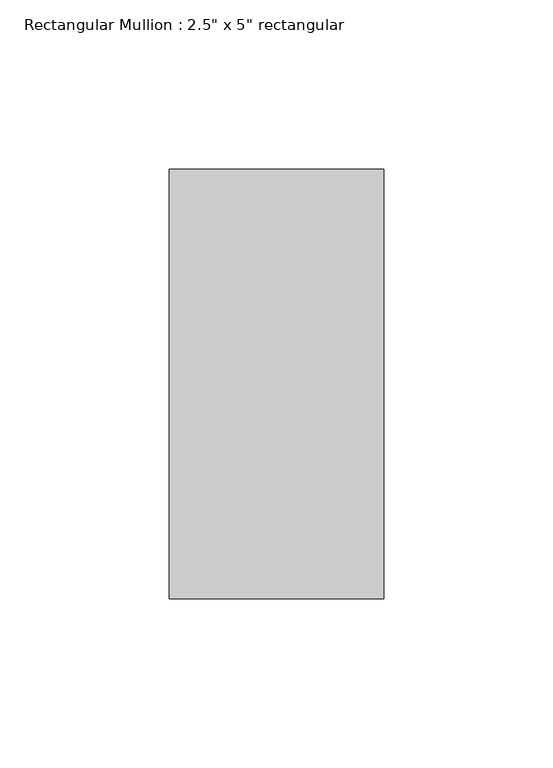
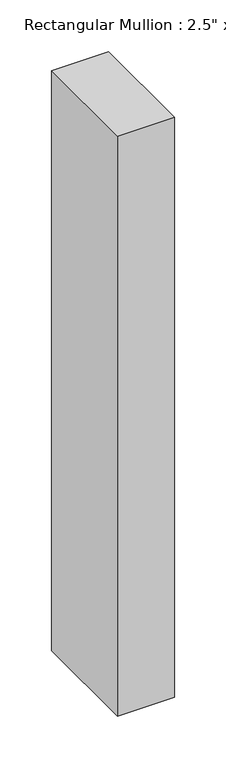
"""IFC4 building model written with IfcOpenShell, lengths in millimetres: member geometry."""

from ifc_helpers import new_model, si_unit, frame, origin, place, context, project, spatial, polyline, outline, extrude, source, transform, mapped, element, save


def member_41a76b6e(model_context):
    return source(origin(), model_context, "Body", "SweptSolid", [
        extrude(outline(polyline([(0.0, 63.5), (0.0, -63.5), (-63.5, -63.5), (-63.5, 63.5), (0.0, 63.5)])), frame((0.0, 0.0, -683.6567525), z_axis=(0.0, 0.0, 1.0), x_axis=(1.0, 0.0, 0.0)), (0.0, 0.0, 1.0), 683.6567525),
    ])


if __name__ == "__main__":
    model = new_model("IFC4")
    model_context = context("Model", 3, world=origin())
    ifc_project = project(units=[si_unit("LENGTHUNIT", "METRE", prefix="MILLI")], contexts=[model_context])
    site = spatial("IfcSite", under=ifc_project)
    building = spatial("IfcBuilding", under=site)
    placement = place(None, origin())
    member_shape = member_41a76b6e(model_context)
    element("IfcMember", 1, ObjectType="Rectangular Mullion : 2.5\" x 5\" rectangular", at=placement, inside=building, context=model_context, shape_type="MappedRepresentation", body=[
        mapped(member_shape, transform((0.0, 0.0, 0.0), x_axis=(1.0, 0.0, 0.0), y_axis=(0.0, 1.0, 0.0), z_axis=(0.0, 0.0, 1.0))),
    ])
    save(model, "model.ifc")

# Revit data of these elements
# Type "Rectangular Mullion : 2.5\" x 5\" rectangular"
#   built-in parameter 1007304 = 0.416667 (stored number, unit not read)
#   built-in parameter 1007301 = 0.104167 (stored number, unit not read)
#   built-in parameter 1007300 = 0.104167 (stored number, unit not read)
# Element 1 (IfcMember, "Rectangular Mullion : 2.5\" x 5\" rectangular")
#   Materials on its faces: "Aluminum"
# Materials
#   "Aluminum": class "Metal", colour RGB 247 247 247, transparency 0, Description = "Aluminum 6061", Cost = 0
